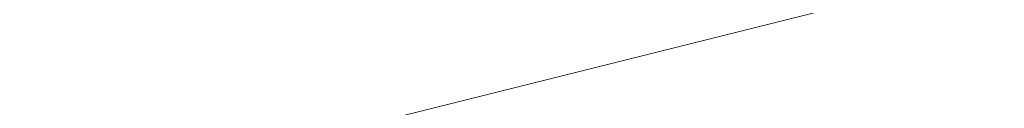
# Model space of a CAD drawing. Units: inches. Extents: x 2091 to 2899, y 967 to 2217.
# Tile 86 of 256: x 2251.278697 to 2251.287593, y 1099.919418 to 1099.920202. Entities that reach past the tile are written whole.
import ezdxf

# ---------------------------------------------------------------- set-up
doc = ezdxf.new("R2010")
doc.units = ezdxf.units.IN
doc.layers.add('A-ANNO-DIMS', color=2, linetype='Continuous', lineweight=18)
doc.layers.add('L-PLNT-TREE', color=94, linetype='Continuous', lineweight=13)
doc.layers.add('A-WALL-PATT', color=141, linetype='Continuous', lineweight=13, true_color=0xadddf7)
doc.styles.get("Standard").update_dxf_attribs({"font": 'arial.ttf'})
doc.dimstyles.new('ISO-25', dxfattribs={"dimtxt": 4, "dimasz": 4, "dimexe": 1.25, "dimexo": 0.625, "dimtad": 1, "dimdec": 0, "dimlunit": 3, "dimtxsty": 'Standard', "dimcen": 2.5, "dimadec": 0, "dimazin": 0, "dimtfac": 1, "dimtdec": 0, "dimtmove": 0, "dimatfit": 3, "dimfxl": 1, "dimarcsym": 0})

# ---------------------------------------------------------------- blocks, each defined once
blk = doc.blocks.new('*U29')
blk.add_line((-402.336, 12.192), (-451.104, 0))
blk = doc.blocks.new('*D71')
at = {"layer": 'A-ANNO-DIMS', "color": 0, "lineweight": -2, "transparency": 16777216}
for p, q in [((2212.143603, 1351.294059), (2212.143603, 969.464303)), ((2452.143603, 1351.294059), (2452.143603, 969.464303)), ((2216.143603, 970.714303), (2448.143603, 970.714303))]:
    blk.add_line(p, q, dxfattribs=at)
at = {"layer": 'A-ANNO-DIMS', "color": 0, "transparency": 16777216}
for points in [[(2216.143603, 971.3809697), (2216.143603, 970.0476363), (2212.143603, 970.714303)], [(2448.143603, 971.3809697), (2448.143603, 970.0476363), (2452.143603, 970.714303)]]:
    blk.add_solid(points, dxfattribs=at)
at = {"layer": 'Defpoints', "color": 0, "transparency": 16777216}
for p in [(2212.143603, 1351.919059), (2452.143603, 1351.919059), (2452.143603, 970.714303)]:
    blk.add_point(p, dxfattribs=at)
at = {"layer": 'A-ANNO-DIMS', "color": 0, "transparency": 16777216, "insert": (2332.143603, 973.381595), "char_height": 4, "attachment_point": 5}
blk.add_mtext('20\'-0"', dxfattribs=at)
blk = doc.blocks.new('*D75')
at = {"layer": 'A-ANNO-DIMS', "color": 0, "lineweight": -2, "transparency": 16777216}
for p, q in [((2212.143603, 1274.794059), (2212.143603, 969.464303)), ((2308.143603, 1274.794059), (2308.143603, 969.464303)), ((2216.143603, 970.714303), (2304.143603, 970.714303))]:
    blk.add_line(p, q, dxfattribs=at)
at = {"layer": 'A-ANNO-DIMS', "color": 0, "transparency": 16777216}
for points in [[(2216.143603, 971.3809697), (2216.143603, 970.0476363), (2212.143603, 970.714303)], [(2304.143603, 971.3809697), (2304.143603, 970.0476363), (2308.143603, 970.714303)]]:
    blk.add_solid(points, dxfattribs=at)
at = {"layer": 'Defpoints', "color": 0, "transparency": 16777216}
for p in [(2212.143603, 1275.419059), (2308.143603, 1275.419059), (2308.143603, 970.714303)]:
    blk.add_point(p, dxfattribs=at)
at = {"layer": 'A-ANNO-DIMS', "color": 0, "transparency": 16777216, "insert": (2260.143603, 973.381595), "char_height": 4, "attachment_point": 5}
blk.add_mtext('8\'-0"', dxfattribs=at)

msp = doc.modelspace()

# ---------------------------------------------------------------- hatches: boundary and pattern name
at = {"layer": 'A-WALL-PATT'}
h = msp.add_hatch(color=256, dxfattribs=at)
h.dxf.hatch_style = 1
h.paths.add_polyline_path([(2803.1436027, 2050.9190588), (2203.1436027, 2050.9190588), (2203.1436027, 1090.9190588), (2803.1436027, 1090.9190588)])
h.paths.add_polyline_path([(2635.7988501, 1147.5404649), (2674.5240524, 1147.5404649, 0.376086), (2678.5296653, 1152.8802017), (2678.5296653, 1159.5564734, 0.333335), (2674.524319, 1163.561846), (2674.524319, 1163.5618504), (2674.524319, 1192.9343904), (2635.8059707, 1192.9343904), (2597.0876225, 1192.9343904), (2597.0876225, 1163.561846, 0.333335), (2593.0822761, 1159.5564734), (2593.0822761, 1152.8802017, 0.376086), (2597.087889, 1147.5404649)], flags=0)
h.paths.add_polyline_path([(2436.0104329, 1278.2407784, 0.000483), (2435.9526433, 1278.215027, -0.001328), (2435.9356253, 1278.1116934, -0.001711), (2436.1164401, 1278.0407583, 0.002185)], flags=0)
h.paths.add_polyline_path([(2794.1436027, 1143.4190588), (2794.1436027, 1347.4190588), (2543.3701706, 1347.4190588), (2543.3701706, 1351.9190588), (2794.1436027, 1351.9190588), (2794.1436027, 1392.7135549), (2793.9473982, 1392.7135549), (2793.9473982, 1473.5368999), (2794.1436027, 1473.5368999), (2794.1436027, 1531.9190588), (2650.1436027, 1531.9190588), (2650.1436027, 1536.4190588), (2794.1436027, 1536.4190588), (2794.1436027, 1692.4190588), (2609.3756095, 1692.4190588), (2609.3756095, 1644.4190588), (2604.8756095, 1644.4190588), (2604.8756095, 1744.9190588), (2609.3756095, 1744.9190588), (2609.3756095, 1696.9190588), (2794.1436027, 1696.9190588), (2794.1436027, 1780.9190588), (2609.6436027, 1780.9190588), (2493.8756095, 1780.9190588), (2493.8756095, 1785.4190588), (2609.6436027, 1785.4190588), (2794.1436027, 1785.4190588), (2794.1436027, 1847.9388214), (2793.9512217, 1847.9388214), (2793.9512217, 1928.7621663), (2794.1436027, 1928.7621663), (2794.1436027, 1941.4190588), (2614.1436027, 1941.4190588), (2614.1436027, 1821.4190588), (2609.6436027, 1821.4190588), (2609.6436027, 1941.4190588), (2392.1436027, 1941.4190588), (2392.1436027, 1819.9190588), (2387.6436027, 1819.9190588), (2387.6436027, 1941.4190588), (2212.1436027, 1941.4190588), (2212.1436027, 1783.9190588), (2392.1436027, 1783.9190588), (2392.1436027, 1780.9190588), (2212.1436027, 1780.9190588), (2212.1436027, 1629.4190588), (2387.6436027, 1629.4190588), (2387.6436027, 1744.9190588), (2392.1436027, 1744.9190588), (2392.1436027, 1627.9190588), (2317.1436027, 1627.9190588), (2317.1436027, 1551.4190588), (2317.1436027, 1536.4190588), (2459.3835909, 1536.4190588), (2459.3835909, 1602.3964802), (2463.8835909, 1602.3964802), (2463.8835909, 1531.9190588), (2456.6436027, 1531.9190588), (2456.6436027, 1529.9190588), (2452.1436027, 1529.9190588), (2452.1436027, 1531.9190588), (2312.6436027, 1531.9190588), (2312.6436027, 1551.4190588), (2306.1436027, 1551.4190588), (2306.1436027, 1555.9190588), (2308.1436027, 1555.9190588), (2308.1436027, 1551.4190588), (2312.6436027, 1551.4190588), (2312.6436027, 1627.9190588), (2212.1436027, 1627.9190588), (2212.1436027, 1555.9190588), (2270.1436027, 1555.9190588), (2270.1436027, 1551.4190588), (2212.1436027, 1551.4190588), (2212.1436027, 1351.9190588), (2272.1436027, 1351.9190588), (2272.1436027, 1347.4190588), (2212.1436027, 1347.4190588), (2212.1436027, 1275.4190588), (2308.1436027, 1275.4190588), (2308.1436027, 1351.9190588), (2452.1436027, 1351.9190588), (2452.1436027, 1493.9190588), (2456.6436027, 1493.9190588), (2456.6436027, 1347.4190588), (2312.6436027, 1347.4190588), (2312.6436027, 1270.9190588), (2212.1436027, 1270.9190588), (2212.1436027, 1099.9190588), (2281.2375229, 1099.9190588), (2282.8710413, 1110.9138034), (2282.0083413, 1116.9966034), (2278.5577413, 1121.4204034), (2268.2056413, 1128.0562034), (2272.0876413, 1128.0562034), (2273.8129413, 1131.9270034), (2279.4203413, 1134.6919034), (2285.0278413, 1135.2449034), (2287.6158413, 1137.4568034), (2288.0471413, 1138.0098034), (2289.3411413, 1140.7747034), (2291.0665413, 1139.6687034), (2292.3605413, 1135.2449034), (2295.3798413, 1136.9038034), (2296.2425413, 1135.7979034), (2297.1052413, 1133.0330034), (2300.1246413, 1138.0098034), (2303.1439413, 1138.0098034), (2304.4379413, 1135.7979034), (2303.1439413, 1133.5860034), (2306.5946413, 1134.6919034), (2307.8887413, 1133.0330034), (2310.9080413, 1135.2449034), (2313.9274413, 1134.1389034), (2315.6268599, 1132.4271023), (2308.3200413, 1117.5496034), (2290.2038413, 1109.8079034), (2288.9098413, 1103.1721034), (2289.2723086, 1099.9190588), (2434.9182274, 1099.9190588), (2431.5932274, 1124.7880588), (2429.9302274, 1169.5530588), (2430.9271848, 1240.5196942), (2435.6589255, 1238.1861258), (2437.1352274, 1196.5540588), (2438.7982274, 1143.9730588), (2442.6782274, 1111.9980588), (2446.5582274, 1099.9190588), (2794.1436027, 1099.9190588), (2794.1436027, 1138.9190588), (2548.0324471, 1138.9190588), (2548.0324471, 1143.4190588), (2548.0324471, 1148.8190588), (2546.6684571, 1148.0315588), (2528.6856919, 1179.1786218, 0.256256), (2512.0324471, 1148.8190588), (2512.0324471, 1143.4190588), (2512.0324471, 1138.9190588), (2507.5324471, 1138.9190588), (2507.5324471, 1143.4190588), (2507.5324471, 1148.8190588, 0.256256), (2490.8792023, 1179.1786218), (2472.8964371, 1148.0315588), (2471.5324471, 1148.8190588), (2471.5324471, 1143.4190588), (2467.0324471, 1143.4190588), (2467.0324471, 1269.9457858, 0.039061), (2460.9099871, 1273.5800588), (2467.0324471, 1273.5800588), (2467.0324471, 1286.3253638, 0.014511), (2465.2161944, 1286.7619052), (2467.0324471, 1287.0525761), (2467.0324471, 1323.4190588), (2471.5324471, 1323.4190588), (2471.5324471, 1148.8190588), (2489.5324471, 1179.9959734), (2490.8964371, 1179.2084734), (2490.8792023, 1179.1786218, -0.256256), (2507.5324471, 1148.8190588), (2507.5324471, 1143.4190588), (2512.0324471, 1143.4190588), (2512.0324471, 1148.8190588, -0.256256), (2528.6856919, 1179.1786218), (2528.6684571, 1179.2084734), (2530.0324471, 1179.9959734), (2548.0324471, 1148.8190588), (2548.0324471, 1143.4190588)], flags=16)
h.paths.add_polyline_path([(2607.7685461, 1200.9450832), (2607.7685461, 1265.0306251), (2597.0876225, 1281.0520106), (2619.7845852, 1281.0520106), (2627.795278, 1337.1268598), (2635.7988501, 1337.1268598), (2643.8166634, 1337.1268598), (2651.8273562, 1281.0520106), (2674.524319, 1281.0520106), (2663.8433953, 1265.0306251), (2663.8433953, 1200.9450832), (2635.8059707, 1200.9450832)], flags=0)
edge = h.paths.add_edge_path(flags=0)
edge.add_ellipse((13303.8962153, 1272.9987247), major_axis=(-10595.3130399, 0.0000005), ratio=0.842303870086, start_angle=0.62823721906, end_angle=0.64655409989, ccw=False)
edge.add_ellipse((2711.7004495, 1156.8526781), major_axis=(2.2197691, 0), ratio=0.84230387, start_angle=111.5352435, end_angle=180.6282372, ccw=False)
edge.add_ellipse((13303.1562922, 1272.9987246), major_axis=(-10593.0263064, 0), ratio=0.842303869544, start_angle=0.52827147182, end_angle=0.64655409706, ccw=False)
edge.add_line((2710.7645961, 1175.3332951), (2710.1299858, 1175.3332951))
edge.add_ellipse((2710.1299858, 1176.5797752), major_axis=(1.4798461, 0), ratio=0.84230387, start_angle=180, end_angle=270, ccw=False)
edge.add_line((2708.6501397, 1176.5797752), (2708.6501397, 1200.7829144))
edge.add_ellipse((2710.1299858, 1200.7829144), major_axis=(1.4798461, 0), ratio=0.84230387, start_angle=90, end_angle=180, ccw=False)
edge.add_line((2710.1299858, 1202.0293944), (2710.4650752, 1202.0293944))
edge.add_ellipse((13303.1562922, 1272.9987246), major_axis=(-10593.0263064, 0), ratio=0.842303869544, start_angle=-0.09022908859, end_angle=0.38386677879, ccw=False)
edge.add_ellipse((2710.1299858, 1290.9270308), major_axis=(-1.4798461, 0), ratio=0.84230387, start_angle=0, end_angle=90, ccw=False)
edge.add_line((2708.6501397, 1290.9270308), (2708.6501397, 1315.13017))
edge.add_ellipse((2710.1299858, 1315.13017), major_axis=(-1.4798461, 0), ratio=0.84230387, start_angle=-90, end_angle=0, ccw=False)
edge.add_line((2710.1299858, 1316.3766501), (2710.7063141, 1316.3766501))
edge.add_ellipse((3238.4017202, 1296.2895655), major_axis=(528.2339998, 0), ratio=0.84230386954, start_angle=176.349572414, end_angle=177.820049686, ccw=False)
edge.add_ellipse((2775.0630432, 1071.4506962), major_axis=(313.3077613, 0), ratio=0.84230386954, start_angle=102.125965552, end_angle=103.780528989, ccw=False)
edge.add_ellipse((2775.0630432, 1078.3056979), major_axis=(-305.3028915, 0), ratio=0.84230386955, start_angle=-79.790461003, end_angle=-77.555372706, ccw=False)
edge.add_ellipse((2695.1417666, 1541.9753825), major_axis=(-250.9602162, 0), ratio=0.84230386954, start_angle=99.256566007, end_angle=102.554932644)
edge.add_line((2741.4103262, 1334.2142554), (2747.1325454, 1337.3784768))
edge.add_ellipse((2747.5386163, 1336.8574776), major_axis=(-0.739923, 0), ratio=0.84230387, start_angle=270, end_angle=307.9331305, ccw=False)
edge.add_ellipse((2747.5386163, 1336.8574776), major_axis=(-0.739923, 0), ratio=0.84230387, start_angle=232.0668695, end_angle=270, ccw=False)
edge.add_line((2747.9446872, 1337.3784768), (2753.6669064, 1334.2142554))
edge.add_ellipse((2799.935466, 1541.9753825), major_axis=(250.9602162, 0), ratio=0.84230386954, start_angle=257.445067356, end_angle=260.743433993)
edge.add_ellipse((2720.0141894, 1078.3056979), major_axis=(305.3028915, 0), ratio=0.84230386954, start_angle=77.555372707, end_angle=79.790461003, ccw=False)
edge.add_ellipse((2720.0141894, 1071.4506962), major_axis=(-313.3077613, 0), ratio=0.84230386954, start_angle=256.219471011, end_angle=257.874034448, ccw=False)
edge.add_ellipse((2256.6755124, 1296.2895655), major_axis=(-528.2339998, 0), ratio=0.84230386954, start_angle=182.179950314, end_angle=183.650427586, ccw=False)
edge.add_line((2784.3709184, 1316.3766501), (2784.9472468, 1316.3766501))
edge.add_ellipse((2784.9472468, 1315.13017), major_axis=(1.4798461, 0), ratio=0.84230387, start_angle=0, end_angle=90, ccw=False)
edge.add_line((2786.4270928, 1315.13017), (2786.4270928, 1290.9270308))
edge.add_ellipse((2784.9472468, 1290.9270308), major_axis=(1.4798461, 0), ratio=0.84230387, start_angle=270, end_angle=360, ccw=False)
edge.add_ellipse((-7808.0790596, 1272.9987246), major_axis=(10593.0263063, 0), ratio=0.842303869544, start_angle=-0.38386677879, end_angle=0.09022908859, ccw=False)
edge.add_line((2784.6121574, 1202.0293944), (2784.9472468, 1202.0293944))
edge.add_ellipse((2784.9472468, 1200.7829144), major_axis=(1.4798461, 0), ratio=0.84230387, start_angle=0, end_angle=90, ccw=False)
edge.add_line((2786.4270928, 1200.7829144), (2786.4270928, 1176.5797752))
edge.add_ellipse((2784.9472468, 1176.5797752), major_axis=(-1.4798461, 0), ratio=0.84230387, start_angle=90, end_angle=180, ccw=False)
edge.add_line((2784.9472468, 1175.3332951), (2784.3126365, 1175.3332951))
edge.add_ellipse((-7808.0790596, 1272.9987246), major_axis=(10593.0263063, 0), ratio=0.842303869544, start_angle=-0.61864319632, end_angle=-0.52827147182, ccw=False)
edge.add_ellipse((2783.3767831, 1156.8526781), major_axis=(-2.2197691, 0), ratio=0.84230387, start_angle=179.3717628, end_angle=248.4647566, ccw=False)
edge.add_ellipse((-7808.8189826, 1272.9987246), major_axis=(-10595.3130398, 0.0000036), ratio=0.842303865762, start_angle=179.3534459226, end_angle=179.37176280343, ccw=False)
edge.add_ellipse((2780.2973026, 1153.500793), major_axis=(-5.2464256, 0), ratio=0.84230387, start_angle=90, end_angle=179.3534459, ccw=False)
edge.add_line((2780.2973026, 1149.0817084), (2714.77993, 1149.0817084))
edge.add_ellipse((2714.77993, 1153.500793), major_axis=(5.2464256, 0), ratio=0.84230387, start_angle=180.6465541, end_angle=270, ccw=False)
edge = h.paths.add_edge_path(flags=0)
edge.add_line((2718.1873674, 1151.0078329), (2718.1873674, 1170.4723638))
edge.add_ellipse((2721.1470595, 1170.4723638), major_axis=(-2.9596921, 0), ratio=0.84230387, start_angle=-90, end_angle=0, ccw=False)
edge.add_line((2721.1470595, 1172.965324), (2773.9301731, 1172.965324))
edge.add_ellipse((2773.9301731, 1170.4723638), major_axis=(-2.9596921, 0), ratio=0.84230387, start_angle=180, end_angle=270, ccw=False)
edge.add_line((2776.8898652, 1170.4723638), (2776.8898652, 1151.0078329))
edge.add_line((2776.8898652, 1151.0078329), (2718.1873674, 1151.0078329))
edge = h.paths.add_edge_path(flags=0)
edge.add_line((2718.1873674, 1180.2341502), (2718.1873674, 1199.0578342))
edge.add_ellipse((2747.5386163, 1320.3986402), major_axis=(147.0179239, 0), ratio=0.84230386954, start_angle=256.40186531, end_angle=283.59813469)
edge.add_line((2776.8898652, 1199.0578342), (2776.8898652, 1180.2341502))
edge.add_ellipse((2747.5386163, 1301.5749562), major_axis=(147.0179239, 0), ratio=0.84230386954, start_angle=256.40186531, end_angle=283.59813469, ccw=False)
edge = h.paths.add_edge_path(flags=0)
edge.add_ellipse((13303.1562922, 1272.9987246), major_axis=(-10591.5464603, 0), ratio=0.842303869555, start_angle=0.05559431352, end_angle=0.37776419393, ccw=False)
edge.add_line((2711.6168595, 1262.7217103), (2715.6674076, 1249.4953957))
edge.add_ellipse((6413.8919626, 1241.691919), major_axis=(-3698.2361592, 0), ratio=0.842303869547, start_angle=-0.120897369, end_angle=0.3640763489)
edge.add_line((2715.7610383, 1218.1924547), (2711.9343065, 1203.167361))
edge = h.paths.add_edge_path(flags=0)
edge.add_line((2718.1873674, 1251.074566), (2716.0024854, 1267.4504351))
edge.add_ellipse((2742.1511746, 1202.1895399), major_axis=(81.7725845, 0), ratio=0.8423038695, start_angle=94.277420963, end_angle=111.834953797, ccw=False)
edge.add_line((2737.0097482, 1270.9306255), (2758.0674844, 1270.9306255))
edge.add_ellipse((2752.926058, 1202.1895399), major_axis=(81.7725845, 0), ratio=0.8423038695, start_angle=68.165046203, end_angle=85.722579037, ccw=False)
edge.add_line((2779.0747472, 1267.4504351), (2776.8898652, 1251.074566))
edge.add_ellipse((2750.3380588, 1187.8853558), major_axis=(79.5796641, 0), ratio=0.8423038695, start_angle=67.208085122, end_angle=85.129930403)
edge.add_line((2756.0346562, 1254.7436557), (2739.0425764, 1254.7436557))
edge.add_ellipse((2744.7391738, 1187.8853558), major_axis=(79.5796641, 0), ratio=0.8423038695, start_angle=94.870069597, end_angle=112.791914878)
edge = h.paths.add_edge_path(flags=0)
edge.add_line((2783.1429261, 1203.167361), (2779.3161943, 1218.1924547))
edge.add_ellipse((-918.81473, 1241.691919), major_axis=(3698.2361592, 0), ratio=0.842303869546, start_angle=-0.3640763489, end_angle=0.120897369)
edge.add_line((2779.409825, 1249.4953957), (2783.4603731, 1262.7217103))
edge.add_ellipse((-7808.0790596, 1272.9987246), major_axis=(-10591.5464603, 0), ratio=0.84230386954, start_angle=179.6222358061, end_angle=179.94440568651, ccw=False)
edge = h.paths.add_edge_path(flags=0)
edge.add_ellipse((2734.2008921, 1286.6904402), major_axis=(-0.3566086, 6.3400775), ratio=0.603833576, start_angle=89.00201428, end_angle=253.65740805, ccw=False)
edge.add_line((2730.3690013, 1286.5418057), (2730.3690013, 1301.3519803))
edge.add_line((2730.3690013, 1301.3519803), (2735.9133107, 1305.2148028))
edge.add_ellipse((2736.3849168, 1304.7345612), major_axis=(0.739923, 0), ratio=0.84230387, start_angle=90, end_angle=134.4802109, ccw=False)
edge.add_line((2736.3849168, 1305.3578013), (2738.0327829, 1305.3578013))
edge.add_line((2738.0327829, 1305.3578013), (2738.0327829, 1307.7079274))
edge.add_ellipse((2794.201642, 1307.7079274), major_axis=(56.168859, 0), ratio=0.8423038695, start_angle=150.5614304, end_angle=180, ccw=False)
edge.add_ellipse((2700.8755906, 1307.7079274), major_axis=(-56.168859, 0), ratio=0.8423038695, start_angle=180, end_angle=209.4385696, ccw=False)
edge.add_line((2757.0444497, 1307.7079274), (2757.0444497, 1305.3578013))
edge.add_line((2757.0444497, 1305.3578013), (2758.6923157, 1305.3578013))
edge.add_ellipse((2758.6923157, 1304.7345612), major_axis=(-0.739923, 0), ratio=0.84230387, start_angle=225.5197891, end_angle=270, ccw=False)
edge.add_line((2759.1639219, 1305.2148028), (2764.7082312, 1301.3519803))
edge.add_line((2764.7082312, 1301.3519803), (2764.7082312, 1286.5418057))
edge.add_ellipse((2760.8763405, 1286.6904402), major_axis=(0.3566086, 6.3400775), ratio=0.603833576, start_angle=106.34259195, end_angle=270.99798572, ccw=False)
edge.add_line((2757.0444497, 1285.7970896), (2757.0444497, 1307.7079274))
edge.add_ellipse((2700.8755906, 1307.7079274), major_axis=(-56.168859, 0), ratio=0.8423038695, start_angle=180, end_angle=209.4385696)
edge.add_ellipse((2794.201642, 1307.7079274), major_axis=(56.168859, 0), ratio=0.8423038695, start_angle=150.5614304, end_angle=180)
edge.add_line((2738.0327829, 1307.7079274), (2738.0327829, 1285.7970896))
h.paths.add_polyline_path([(2417.8122727, 1104.449704), (2413.4922727, 1102.529704), (2410.6122727, 1103.969704), (2409.1722727, 1106.369704), (2407.2522727, 1107.329704), (2406.2922727, 1109.729704), (2405.3322727, 1114.049704), (2405.3322727, 1117.889704), (2406.2922727, 1120.129704), (2407.2522727, 1119.809704), (2408.8483218, 1118.3276585), (2410.1739451, 1119.4241703), (2410.2112727, 1120.405704), (2411.0407305, 1121.4190541), (2410.6992727, 1119.858704), (2410.1739451, 1119.4241703), (2410.0884515, 1117.1761095), (2411.1328361, 1116.2063237), (2413.9722727, 1119.329704), (2416.8522727, 1120.769704), (2416.8697209, 1120.7987842), (2417.0350713, 1119.4051162), (2417.8962134, 1118.1433844), (2418.2922727, 1118.369704), (2419.5444467, 1120.0392692), (2419.3609153, 1118.387487), (2419.0321078, 1119.3561507), (2418.3989394, 1118.5119262), (2419.2522727, 1114.529704), (2418.7940909, 1107.1987949)], flags=0)
h.paths.add_polyline_path([(2508.8701706, 1347.4190588), (2508.3701706, 1347.4190588), (2508.3701706, 1351.9190588), (2508.8701706, 1351.9190588)], flags=0)
h.paths.add_polyline_path([(2473.3701706, 1347.4190588), (2472.3701706, 1347.4190588), (2467.8701706, 1347.4190588), (2467.8701706, 1455.4190588), (2472.3701706, 1455.4190588), (2472.3701706, 1352.4190588), (2473.3701706, 1352.4190588)], flags=0)
h.paths.add_polyline_path([(2352.106244, 1217.4461971), (2349.226244, 1218.8861971), (2347.786244, 1221.2861971), (2345.866244, 1222.2461971), (2344.906244, 1224.6461971), (2343.946244, 1228.9661971), (2343.946244, 1232.8061971), (2344.906244, 1235.0461971), (2345.866244, 1234.7261971), (2347.4622931, 1233.2441515), (2348.7879164, 1234.3406634), (2348.825244, 1235.3221971), (2349.6547018, 1236.3355471), (2349.313244, 1234.7751971), (2348.7879164, 1234.3406634), (2348.7024228, 1232.0926025), (2349.7468074, 1231.1228168), (2352.586244, 1234.2461971), (2355.466244, 1235.6861971), (2355.4836921, 1235.7152773), (2355.6490426, 1234.3216093), (2356.5101846, 1233.0598774), (2356.906244, 1233.2861971), (2358.1584179, 1234.9557623), (2357.9748866, 1233.3039801), (2357.6460791, 1234.2726438), (2357.0129107, 1233.4284193), (2357.866244, 1229.4461971), (2357.4080622, 1222.115288), (2356.426244, 1219.3661971)], flags=0)
h.paths.add_polyline_path([(2348.2967999, 1112.2244204), (2347.0137999, 1112.3104204), (2345.5297999, 1114.1274204), (2345.7317999, 1115.8584204), (2346.8117999, 1116.9824204), (2346.8117999, 1114.6464204), (2345.8667999, 1114.2144204), (2346.8797999, 1114.3004204)], flags=0)
h.paths.add_polyline_path([(2347.0137999, 1110.9264204), (2346.2717999, 1110.4934204), (2346.6097999, 1111.1864204)], flags=0)
h.paths.add_polyline_path([(2345.8667999, 1118.1944204), (2345.5297999, 1117.3294204), (2343.7077999, 1118.0214204), (2344.3827999, 1118.6264204)], flags=0)
h.paths.add_polyline_path([(2346.6767999, 1109.2824204), (2346.0697999, 1108.0714204), (2345.8667999, 1110.0614204)], flags=0)
h.paths.add_polyline_path([(2345.0567999, 1119.7514204), (2343.6397999, 1119.7514204), (2343.9777999, 1121.1354204)], flags=0)
h.paths.add_polyline_path([(2345.2597999, 1116.5504204), (2345.1247999, 1115.8584204), (2344.9217999, 1115.6854204), (2344.7197999, 1116.3774204)], flags=0)
h.paths.add_polyline_path([(2345.6647999, 1112.3104204), (2345.4617999, 1111.5324204), (2344.0447999, 1111.9644204), (2344.6517999, 1112.5704204)], flags=0)
h.paths.add_polyline_path([(2345.1917999, 1113.3494204), (2344.4497999, 1113.8684204), (2344.7197999, 1114.3874204)], flags=0)
h.paths.add_polyline_path([(2344.6517999, 1116.8094204), (2344.1797999, 1115.6854204), (2344.6517999, 1115.3394204), (2343.9097999, 1114.9064204), (2343.0327999, 1115.9444204), (2343.6397999, 1116.4634204)], flags=0)
h.paths.add_polyline_path([(2345.8667999, 1106.6864204), (2344.9897999, 1105.5624204), (2344.5167999, 1106.6004204)], flags=0)
h.paths.add_polyline_path([(2344.8547999, 1110.0614204), (2344.5167999, 1109.2824204), (2344.1127999, 1109.7154204)], flags=0)
h.paths.add_polyline_path([(2344.0447999, 1113.5224204), (2343.4377999, 1113.0894204), (2342.7627999, 1113.9544204)], flags=0)
h.paths.add_polyline_path([(2344.3147999, 1111.0124204), (2342.9647999, 1110.3204204), (2342.9647999, 1111.0994204)], flags=0)
h.paths.add_polyline_path([(2345.1247999, 1104.6974204), (2344.5847999, 1103.7454204), (2344.4497999, 1104.2644204)], flags=0)
h.paths.add_polyline_path([(2342.8297999, 1121.2224204), (2341.7497999, 1120.5304204), (2340.5357999, 1121.0494204), (2340.1307999, 1121.8284204), (2340.6707999, 1122.9524204), (2341.1427999, 1121.8284204), (2341.6147999, 1122.0014204)], flags=0)
h.paths.add_polyline_path([(2342.9647999, 1119.7514204), (2343.0327999, 1118.4534204), (2342.0877999, 1118.0214204), (2342.0197999, 1119.4914204)], flags=0)
h.paths.add_polyline_path([(2342.6947999, 1116.8964204), (2341.9527999, 1116.6364204), (2342.0197999, 1117.3294204)], flags=0)
h.paths.add_polyline_path([(2343.0327999, 1112.2244204), (2342.0197999, 1111.7914204), (2341.5477999, 1112.2244204), (2342.3577999, 1113.3494204)], flags=0)
h.paths.add_polyline_path([(2343.7747999, 1104.4374204), (2342.6277999, 1102.8804204), (2342.6947999, 1104.6104204), (2343.4377999, 1105.1294204)], flags=0)
h.paths.add_polyline_path([(2342.0197999, 1115.0794204), (2340.8057999, 1115.5124204), (2340.9407999, 1116.3774204)], flags=0)
h.paths.add_polyline_path([(2341.4807999, 1120.0974204), (2341.4807999, 1119.4054204), (2341.0757999, 1119.5784204), (2341.1427999, 1120.0974204)], flags=0)
h.paths.add_polyline_path([(2341.8177999, 1114.4734204), (2340.9407999, 1113.0894204), (2340.8057999, 1114.5604204)], flags=0)
h.paths.add_polyline_path([(2341.1427999, 1118.5404204), (2340.9407999, 1116.9824204), (2339.0507999, 1117.6754204), (2339.0507999, 1118.6264204)], flags=0)
h.paths.add_polyline_path([(2342.6947999, 1101.6684204), (2341.9527999, 1101.8414204), (2342.5597999, 1102.3614204)], flags=0)
h.paths.add_polyline_path([(2340.3327999, 1119.6654204), (2338.4437999, 1119.5784204), (2337.9037999, 1120.3574204), (2339.6577999, 1120.6164204)], flags=0)
h.paths.add_polyline_path([(2340.3327999, 1115.3394204), (2340.0627999, 1113.6954204), (2339.3877999, 1115.3394204)], flags=0)
h.paths.add_polyline_path([(2341.8177999, 1103.8314204), (2341.5477999, 1102.8804204), (2341.1427999, 1103.6584204)], flags=0)
h.paths.add_polyline_path([(2339.0507999, 1122.8664204), (2337.2957999, 1121.8284204), (2337.0937999, 1123.1254204), (2337.7687999, 1123.8184204)], flags=0)
h.paths.add_polyline_path([(2339.1177999, 1121.7414204), (2338.8477999, 1121.2224204), (2338.1737999, 1121.0494204), (2338.3757999, 1121.5684204)], flags=0)
h.paths.add_polyline_path([(2339.1857999, 1119.3194204), (2338.6457999, 1118.7134204), (2338.2407999, 1118.1074204), (2338.2407999, 1118.8864204)], flags=0)
h.paths.add_polyline_path([(2341.1427999, 1101.9284204), (2340.6027999, 1101.2364204), (2340.0627999, 1101.8414204), (2340.6027999, 1102.3614204)], flags=0)
h.paths.add_polyline_path([(2337.6337999, 1117.7614204), (2336.6207999, 1118.2804204), (2337.2957999, 1118.9724204)], flags=0)
h.paths.add_polyline_path([(2336.8237999, 1119.5784204), (2334.7987999, 1118.9724204), (2335.2037999, 1120.3574204), (2336.5537999, 1120.8764204)], flags=0)
h.paths.add_polyline_path([(2339.1177999, 1100.4574204), (2337.3637999, 1100.5434204), (2336.7557999, 1101.2364204)], flags=0)
h.paths.add_polyline_path([(2336.3507999, 1122.4334204), (2336.0137999, 1121.9144204), (2334.9337999, 1122.4334204), (2334.5287999, 1123.4714204), (2335.7437999, 1122.7794204)], flags=0)
h.paths.add_polyline_path([(2334.7317999, 1120.8764204), (2334.2587999, 1120.3574204), (2334.0567999, 1120.7894204), (2334.5967999, 1121.3084204)], flags=0)
h.paths.add_polyline_path([(2334.4617999, 1122.1744204), (2332.5717999, 1121.3084204), (2331.3567999, 1122.1744204), (2332.0997999, 1122.8664204)], flags=0)
h.paths.add_polyline_path([(2334.2587999, 1118.5404204), (2333.3817999, 1118.4534204), (2333.6517999, 1119.3194204)], flags=0)
h.paths.add_polyline_path([(2335.5417999, 1102.2744204), (2334.1917999, 1102.6204204), (2335.2717999, 1103.3124204)], flags=0)
h.paths.add_polyline_path([(2332.7067999, 1119.6654204), (2331.6947999, 1120.4434204), (2332.5047999, 1120.7894204)], flags=0)
h.paths.add_polyline_path([(2334.7317999, 1101.1494204), (2333.5167999, 1101.5824204), (2333.9887999, 1101.7554204)], flags=0)
h.paths.add_polyline_path([(2332.6397999, 1116.6364204), (2331.0867999, 1116.2904204), (2331.9647999, 1118.1944204)], flags=0)
h.paths.add_polyline_path([(2330.7497999, 1121.5684204), (2330.2767999, 1120.2704204), (2328.5227999, 1119.3194204), (2328.9947999, 1121.0494204)], flags=0)
h.paths.add_polyline_path([(2330.7497999, 1118.6264204), (2330.0077999, 1117.5024204), (2329.8727999, 1118.0214204)], flags=0)
h.paths.add_polyline_path([(2332.0997999, 1102.3614204), (2330.5467999, 1102.0144204), (2331.6947999, 1102.9664204)], flags=0)
h.paths.add_polyline_path([(2329.5347999, 1113.6084204), (2329.0627999, 1112.3104204), (2328.5897999, 1113.3494204)], flags=0)
h.paths.add_polyline_path([(2328.3877999, 1117.8484204), (2327.5097999, 1116.5504204), (2327.1727999, 1117.7614204)], flags=0)
h.paths.add_polyline_path([(2329.7377999, 1106.5134204), (2329.5347999, 1105.3024204), (2328.2527999, 1106.0814204)], flags=0)
h.paths.add_polyline_path([(2328.6577999, 1114.3874204), (2328.0497999, 1114.1274204), (2328.3197999, 1114.9064204)], flags=0)
h.paths.add_polyline_path([(2328.3197999, 1112.2244204), (2327.1057999, 1112.1374204), (2326.7007999, 1112.6564204)], flags=0)
h.paths.add_polyline_path([(2326.9027999, 1115.2524204), (2326.7007999, 1114.1274204), (2325.2157999, 1113.6084204), (2326.0927999, 1115.3394204)], flags=0)
h.paths.add_polyline_path([(2326.6327999, 1108.3304204), (2326.0927999, 1107.3794204), (2325.8907999, 1108.5034204), (2326.4977999, 1109.1094204)], flags=0)
h.paths.add_polyline_path([(2615.1436027, 1531.9190588), (2609.6436027, 1531.9190588), (2609.6436027, 1620.4190588), (2614.1436027, 1620.4190588), (2614.1436027, 1536.4190588), (2615.1436027, 1536.4190588)], flags=0)
h.paths.add_polyline_path([(2545.1436027, 1563.4190588), (2464.1436027, 1563.4190588), (2464.1436027, 1632.4190588), (2509.1436027, 1632.4190588), (2509.1436027, 1627.9190588), (2509.1436027, 1603.9190588), (2468.6436027, 1603.9190588), (2468.6436027, 1567.9190588), (2540.6436027, 1567.9190588), (2540.6436027, 1591.9190588), (2545.1436027, 1591.9190588)], flags=0)
h.paths.add_polyline_path([(2388.9690483, 1549.985735), (2357.4341811, 1549.985735), (2357.4341811, 1623.3607783), (2399.3627772, 1623.3607783), (2435.6894654, 1623.3607783), (2435.5925469, 1602.5592734), (2435.5925469, 1602.3964802), (2388.9690483, 1602.3964802)], flags=0)
h.paths.add_polyline_path([(2388.8806282, 1555.8091511), (2374.9044295, 1555.8091511), (2374.9044295, 1600.5715641), (2374.9044295, 1615.4576454), (2406.3508766, 1615.4576454), (2406.3508766, 1618.9394309), (2412.1742927, 1615.4576454), (2406.3508766, 1611.9758599), (2406.3508766, 1615.4576454), (2388.8806282, 1615.4576454)], flags=0)
h.paths.add_polyline_path([(2568.8756095, 1644.4190588), (2453.3756095, 1644.4190588), (2453.3756095, 1785.4190588), (2457.8756095, 1785.4190588), (2457.8756095, 1648.9190588), (2568.8756095, 1648.9190588)], flags=0)
h.paths.add_polyline_path([(2212.1436027, 1945.9190588), (2212.1436027, 2041.9190588), (2794.1436027, 2041.9190588), (2794.1436027, 1945.9190588)], flags=16)
h.paths.add_polyline_path([(2271.0827276, 1964.3172377), (2776.852968, 1964.3172377), (2776.852968, 2037.1696226), (2271.0827276, 2037.1696226)], flags=8)
h.paths.add_polyline_path([(2380.6492852, 1536.8241435), (2461.0408087, 1536.8241435), (2461.0408087, 1554.6525871), (2380.6492852, 1554.6525871)], flags=8)
h.paths.add_polyline_path([(2240.7557092, 1609.7254508), (2309.1858294, 1609.7254508), (2309.1858294, 1617.6982037), (2240.7557092, 1617.6982037)], flags=8)
h.paths.add_polyline_path([(2212.6772554, 1313.5041021), (2282.5915203, 1313.5041021), (2282.5915203, 1322.7452389), (2212.6772554, 1322.7452389)], flags=8)
h.paths.add_polyline_path([(2457.111976, 1114.778574), (2558.4815807, 1114.778574), (2558.4815807, 1142.2196823), (2457.111976, 1142.2196823)], flags=8)
h.paths.add_polyline_path([(2473.4423372, 1273.0100672), (2604.6412257, 1273.0100672), (2604.6412257, 1318.3469349), (2473.4423372, 1318.3469349)], flags=8)
h.paths.add_polyline_path([(2638.8763024, 1626.9774316), (2684.2503675, 1627.9767377), (2684.0384825, 1637.5974944), (2638.6644174, 1636.5981884)], flags=8)
h.paths.add_polyline_path([(2537.5905538, 1453.7934466), (2628.3895472, 1453.7934466), (2628.3895472, 1475.3448114), (2537.5905538, 1475.3448114)], flags=8)
h.paths.add_polyline_path([(2504.1376376, 1714.6323972), (2554.6471875, 1714.6323972), (2554.6471875, 1730.2377115), (2504.1376376, 1730.2377115)], flags=8)
h.paths.add_polyline_path([(2487.5011806, 1575.6518716), (2535.0971214, 1575.6518716), (2535.0971214, 1598.3776456), (2487.5011806, 1598.3776456)], flags=8)
h.paths.add_polyline_path([(2709.0994004, 1735.7102784), (2740.0166009, 1735.7102784), (2740.0166009, 1749.9376406), (2709.0994004, 1749.9376406)], flags=8)
h.paths.add_polyline_path([(2442.4384239, 1792.1716575), (2564.7288353, 1792.1716575), (2564.7288353, 1842.0001626), (2442.4384239, 1842.0001626)], flags=8)
h.paths.add_polyline_path([(2655.8158012, 1809.6440763), (2789.5201425, 1806.6937963), (2790.0849768, 1832.2916379), (2656.3806355, 1835.2419179)], flags=8)
h.paths.add_polyline_path([(2234.8426972, 1797.7201432), (2368.5928512, 1794.7688523), (2369.1607182, 1820.504132), (2235.4105642, 1823.4554229)], flags=8)
h.paths.add_polyline_path([(2245.1384659, 1644.0063348), (2398.4277329, 1640.6238997), (2398.9948417, 1666.3248199), (2245.7055747, 1669.7072549)], flags=8)
h.paths.add_polyline_path([(2306.1428474, 1431.1685186), (2413.7683138, 1428.7936873), (2414.3331481, 1454.3915289), (2306.7076817, 1456.7663602)], flags=8)
h.paths.add_polyline_path([(2306.834582, 1458.2331447), (2393.3804836, 1456.3234487), (2393.9328082, 1481.3543583), (2307.3869066, 1483.2640542)], flags=8)

# ---------------------------------------------------------------- block references
at = {"layer": 'L-PLNT-TREE', "xscale": 0.0393700787401575, "yscale": 0.0393700787401575, "zscale": 0.0393700787401575}
msp.add_blockref('*U29', (2269.0410136, 1099.9190588), dxfattribs=at)

# ---------------------------------------------------------------- dimensions: what is measured, and where the dimension line sits
at = {"layer": 'A-ANNO-DIMS'}
for base, p1, p2, picture, middle in [((2452.143603, 970.714303), (2212.143603, 1351.919059), (2452.143603, 1351.919059), '*D71', (2332.143603, 973.381595)), ((2308.143603, 970.714303), (2212.143603, 1275.419059), (2308.143603, 1275.419059), '*D75', (2260.143603, 973.381595))]:
    dim = msp.add_linear_dim(base=base, p1=p1, p2=p2, dimstyle='ISO-25', override={"dimdec": 1, "dimlfac": 1, "dimrnd": 0, "dimzin": 1, "dimdsep": 46, "dimlunit": 4, "dimfrac": 2}, dxfattribs=at)
    dim.commit()
    dim.dimension.update_dxf_attribs({"geometry": picture, "text_midpoint": middle})

doc.saveas('drawing.dxf')
